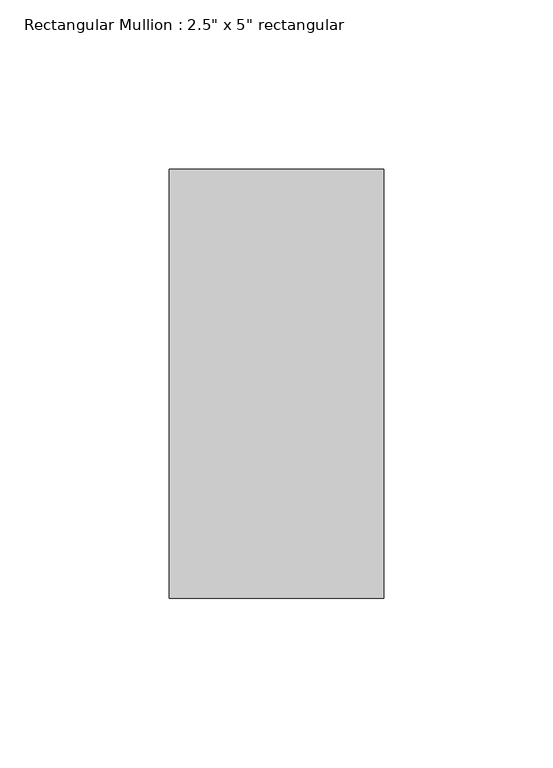
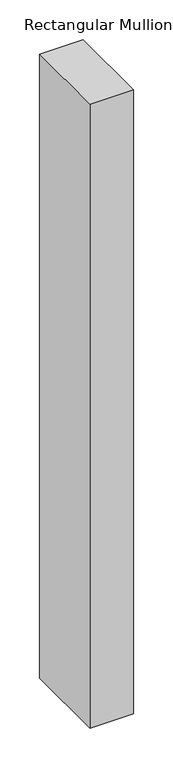
"""IFC4 building model written with IfcOpenShell, lengths in millimetres: member geometry."""

from ifc_helpers import new_model, si_unit, frame, origin, place, context, project, spatial, polyline, outline, extrude, source, transform, mapped, element, save


def member_dd4241ee(model_context):
    return source(origin(), model_context, "Body", "SweptSolid", [
        extrude(outline(polyline([(0.0, 63.5), (0.0, -63.5), (-63.5, -63.5), (-63.5, 63.5), (0.0, 63.5)])), frame((0.0, 0.0, -960.8037122), z_axis=(0.0, 0.0, 1.0), x_axis=(1.0, 0.0, 0.0)), (0.0, 0.0, 1.0), 960.8037122),
    ])


if __name__ == "__main__":
    model = new_model("IFC4")
    model_context = context("Model", 3, world=origin())
    ifc_project = project(units=[si_unit("LENGTHUNIT", "METRE", prefix="MILLI")], contexts=[model_context])
    site = spatial("IfcSite", under=ifc_project)
    building = spatial("IfcBuilding", under=site)
    placement = place(None, origin())
    member_shape = member_dd4241ee(model_context)
    element("IfcMember", 1, ObjectType="Rectangular Mullion : 2.5\" x 5\" rectangular", at=placement, inside=building, context=model_context, shape_type="MappedRepresentation", body=[
        mapped(member_shape, transform((0.0, 0.0, 0.0), x_axis=(1.0, 0.0, 0.0), y_axis=(0.0, 1.0, 0.0), z_axis=(0.0, 0.0, 1.0))),
    ])
    save(model, "model.ifc")

# Revit data of these elements
# Type "Rectangular Mullion : 2.5\" x 5\" rectangular"
#   built-in parameter 1007304 = 0.416667 (stored number, unit not read)
#   built-in parameter 1007301 = 0.104167 (stored number, unit not read)
#   built-in parameter 1007300 = 0.104167 (stored number, unit not read)
# Element 1 (IfcMember, "Rectangular Mullion : 2.5\" x 5\" rectangular")
#   Materials on its faces: "Aluminum"
# Materials
#   "Aluminum": class "Metal", colour RGB 247 247 247, transparency 0, Description = "Aluminum 6061", Cost = 0
